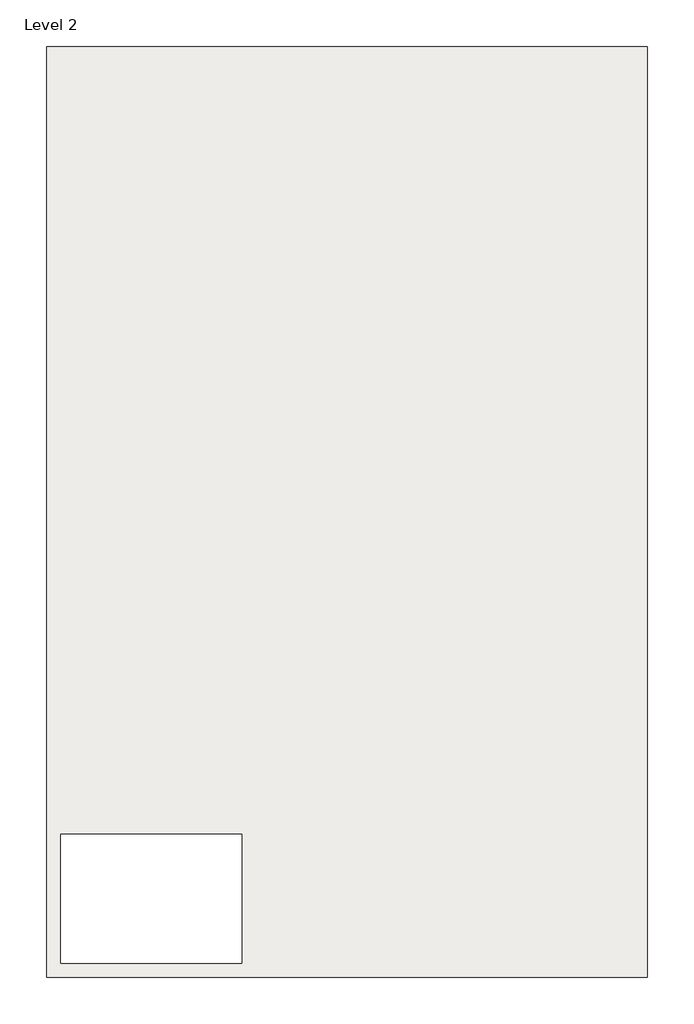
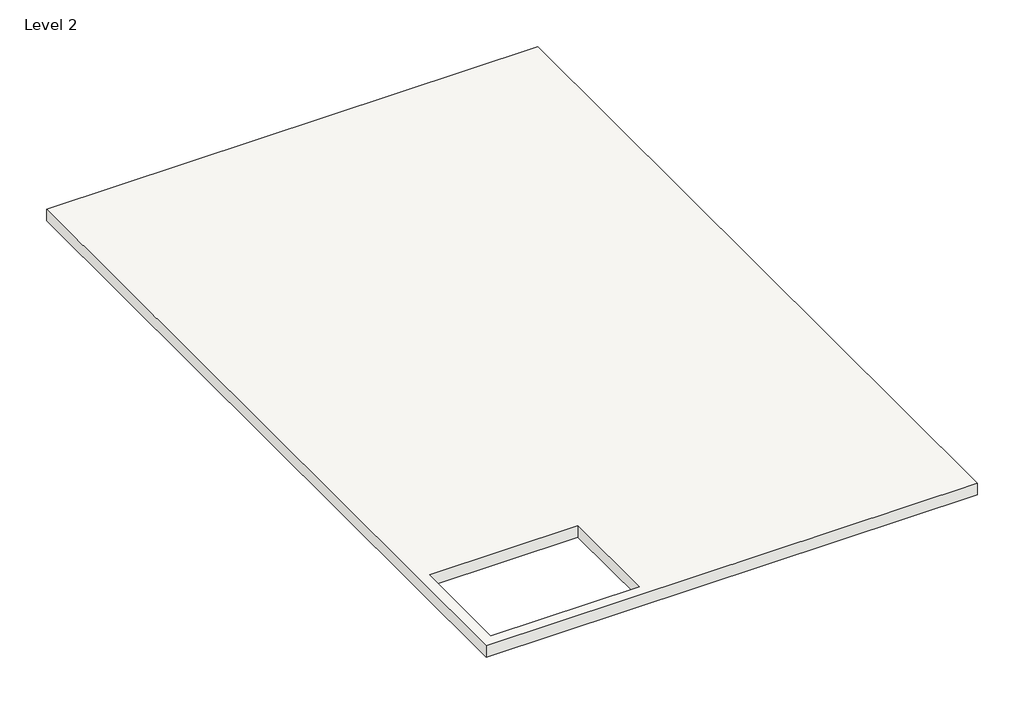
# One storey: 1 roof.
"""IFC4 building model written with IfcOpenShell, lengths in millimetres."""

from ifc_helpers import new_model, si_unit, frame, origin, place, context, project, spatial, polyline, outline, extrude, element, save

model = new_model("IFC4")

# Units and contexts
model_context = context("Model", 3, world=origin())
ifc_project = project(units=[si_unit("LENGTHUNIT", "METRE", prefix="MILLI")], contexts=[model_context])

# Site, building, storey
site = spatial("IfcSite", under=ifc_project)
building = spatial("IfcBuilding", under=site)
storey = spatial("IfcBuildingStorey", under=building, Name="Level 2", Elevation=3048.0)

# Roof
placement = place(None, origin())
element("IfcRoof", 1, ObjectType="Wood Rafter 8\" - Asphalt Shingle - Insulated", at=placement, inside=storey, context=model_context, shape_type="SweptSolid", body=[
    extrude(outline(polyline([(-480.8653968, -1308.9702467), (-9218.4653968, -1308.9702467), (-9218.4653968, 12229.2297533), (-480.8653968, 12229.2297533), (-480.8653968, -1308.9702467)]), holes=[polyline([(-9015.2653968, -1105.7702467), (-6381.8994015, -1105.7702467), (-6381.8994015, 773.8297533), (-9015.2653968, 773.8297533), (-9015.2653968, -1105.7702467)])]), frame((0.0, 0.0, 3048.0), z_axis=(0.0, 0.0, 1.0), x_axis=(1.0, 0.0, 0.0)), (0.0, 0.0, 1.0), 212.725),
])

save(model, "model.ifc")

# Revit data of these elements
# Type "Wood Rafter 8\" - Asphalt Shingle - Insulated"
#   Assembly Code = "B1020"
#   Layers, outside or top first: 0' - 0 1/4" "Asphalt Shingle" (function 4); 0' - 0 5/8" "Plywood, Sheathing" (function 2); 0' - 7 1/2" "Structure, Wood Joist/Rafter Layer, Batt Insulation" (function 1)
# Element 1 (IfcRoof, "Wood Rafter 8\" - Asphalt Shingle - Insulated")
#   built-in parameter 1001705 = 10.6979 (stored number, unit not read)
#   built-in parameter 1001710 = 33615
#   Phase Created = New Construction
#   Materials on its faces: "Structure, Wood Joist/Rafter Layer, Batt Insulation", "Asphalt Shingle"
# Materials
#   "Asphalt Shingle": class "Generic", colour RGB 155 155 155, transparency 0, Description = "Asphalt roofing shingle", Cost = 0
#   "Plywood, Sheathing": class "Wood", colour RGB 212 179 113, transparency 0, Description = "Plywood, sheathing grade", Cost = 0
#   "Structure, Wood Joist/Rafter Layer, Batt Insulation": class "Wood", colour RGB 127 127 127, transparency 0, Description = "Wood framing, insulated", Cost = 0
